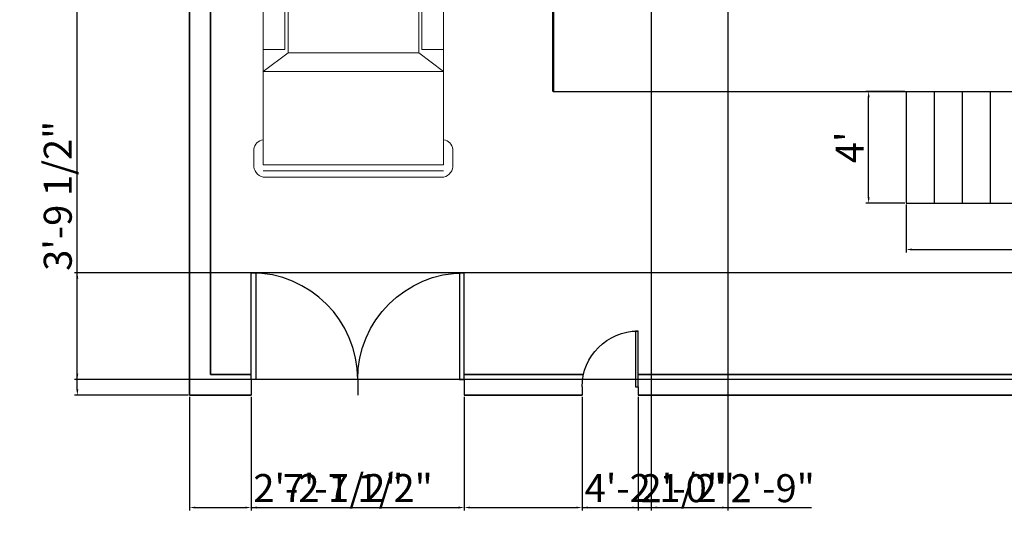
# Model space of a CAD drawing. Units: inches. Extents: x 6286 to 7213, y 5725 to 6776.
# Tile 1 of 5: x 6286 to 6709, y 5725 to 5946. Entities that reach past the tile are written whole.
import ezdxf

# ---------------------------------------------------------------- set-up
doc = ezdxf.new("R2010")
doc.units = ezdxf.units.IN
for name, color, linetype, lineweight in [('A-ANNO-DIMS', 2, 'Continuous', 18), ('A-FLOR', 7, 'Continuous', 25), ('A-FLOR-STRS', 7, 'Continuous', 25), ('A-WALL', 7, 'Continuous', 50), ('C-PKNG-VEHI', 8, 'Continuous', 13), ('C-PROP', 7, 'Continuous', 35), ('L-SITE-GATE', 3, 'Continuous', 25)]:
    doc.layers.add(name, color=color, linetype=linetype, lineweight=lineweight)
doc.styles.get("Standard").update_dxf_attribs({"font": 'arial.ttf'})
doc.dimstyles.new('ISO-25', dxfattribs={"dimtxt": 12, "dimasz": 2.5, "dimexe": 1.25, "dimexo": 0.625, "dimtad": 1, "dimdec": 1, "dimlunit": 4, "dimtxsty": 'Standard', "dimcen": 2.5, "dimadec": 0, "dimazin": 0, "dimtfac": 1, "dimtdec": 1, "dimtmove": 0, "dimatfit": 3, "dimfxl": 1, "dimarcsym": 0})

# ---------------------------------------------------------------- blocks, each defined once
blk = doc.blocks.new('*D19')
at = {"layer": 'A-ANNO-DIMS', "color": 0, "lineweight": -2, "transparency": 16777216}
for p, q in [((6665.8, 5915.26), (6649.05, 5915.26)), ((6650.3, 5869.76), (6650.3, 5912.76)), ((6665.8, 5867.26), (6649.05, 5867.26))]:
    blk.add_line(p, q, dxfattribs=at)
at = {"layer": 'A-ANNO-DIMS', "color": 0, "lineweight": 100, "transparency": 16777216}
for points in [[(6649.89, 5912.76), (6650.72, 5912.76), (6650.3, 5915.26)], [(6649.89, 5869.76), (6650.72, 5869.76), (6650.3, 5867.26)]]:
    blk.add_solid(points, dxfattribs=at)
at = {"layer": 'Defpoints', "color": 0, "lineweight": 100, "transparency": 16777216}
for p in [(6650.3, 5915.26), (6666.42, 5915.26), (6666.42, 5867.26)]:
    blk.add_point(p, dxfattribs=at)
at = {"layer": 'A-ANNO-DIMS', "color": 0, "transparency": 16777216, "insert": (6643.68, 5891.26), "char_height": 12, "attachment_point": 5, "rotation": 90}
blk.add_mtext("4'", dxfattribs=at)
blk = doc.blocks.new('*D20')
at = {"layer": 'A-ANNO-DIMS', "color": 0, "lineweight": -2, "transparency": 16777216}
for p, q in [((6666.42, 5866.64), (6666.42, 5846.12)), ((6882.42, 5866.64), (6882.42, 5846.12)), ((6668.92, 5847.37), (6879.92, 5847.37))]:
    blk.add_line(p, q, dxfattribs=at)
at = {"layer": 'A-ANNO-DIMS', "color": 0, "lineweight": 100, "transparency": 16777216}
for points in [[(6668.92, 5847.78), (6668.92, 5846.95), (6666.42, 5847.37)], [(6879.92, 5847.78), (6879.92, 5846.95), (6882.42, 5847.37)]]:
    blk.add_solid(points, dxfattribs=at)
at = {"layer": 'Defpoints', "color": 0, "lineweight": 100, "transparency": 16777216}
for p in [(6666.42, 5867.26), (6882.42, 5867.26), (6882.42, 5847.37)]:
    blk.add_point(p, dxfattribs=at)
at = {"layer": 'A-ANNO-DIMS', "color": 0, "transparency": 16777216, "insert": (6774.42, 5854.12), "char_height": 12, "attachment_point": 5}
blk.add_mtext("18'", dxfattribs=at)
blk = doc.blocks.new('*U28')
for p, q in [((5.44, 42.31), (12.12, 42.31)), ((189.69, 42.31), (183.01, 42.31)), ((0.1, -0.41), (0.1, 38.35)), ((2.77, -0.41), (2.77, 38.31)), ((5.44, -0.41), (5.44, 38.24)), ((5.45, 38.31), (16.12, 38.31)), ((16.12, 38.31), (180.34, 38.31)), ((61.52, -0.41), (61.52, 38.31)), ((61.52, 38.31), (77.54, 27.62)), ((64.19, 38.31), (76.2, 30.29)), ((76.2, 30.29), (76.2, 38.31)), ((78.87, 38.31), (78.87, 28.96)), ((106.91, 28.96), (106.91, 38.31)), ((109.58, 27.62), (109.58, 38.31)), ((112.25, 38.31), (112.25, 28.96)), ((140.29, 28.96), (140.29, 38.31)), ((141.62, 27.62), (149.64, 38.31)), ((149.64, -0.41), (149.64, 38.31)), ((189.69, 38.31), (179.01, 38.31)), ((189.69, -0.41), (189.69, 38.24)), ((192.36, -0.41), (192.36, 38.31)), ((195.03, -0.41), (195.03, 38.35)), ((77.54, 27.62), (141.62, 27.62)), ((77.54, -0.41), (77.54, 27.62)), ((78.87, 28.96), (106.91, 28.96)), ((112.25, 28.96), (140.29, 28.96)), ((141.62, -0.41), (141.62, 27.62)), ((5.44, 7.6), (61.52, 15.61)), ((0.1, -0.42), (0.1, -39.18)), ((2.77, -0.41), (2.77, -39.13)), ((5.44, -0.42), (5.44, -39.07)), ((61.52, -0.41), (61.52, -39.13)), ((77.54, -0.41), (77.54, -28.45)), ((141.62, -0.41), (141.62, -28.45)), ((149.64, -0.41), (149.64, -39.13)), ((189.69, -0.42), (189.69, -39.07)), ((192.36, -0.41), (192.36, -39.13)), ((195.03, -0.42), (195.03, -39.18)), ((5.44, -8.42), (61.52, -16.43)), ((61.52, -39.13), (77.54, -28.45)), ((77.54, -28.45), (141.62, -28.45)), ((109.58, -28.45), (109.58, -39.13)), ((141.62, -28.45), (149.64, -39.13)), ((64.19, -39.13), (76.2, -31.12)), ((76.2, -31.12), (76.2, -39.13)), ((78.87, -39.13), (78.87, -29.79)), ((78.87, -29.79), (106.91, -29.79)), ((106.91, -29.79), (106.91, -39.13)), ((112.25, -29.79), (140.29, -29.79)), ((112.25, -39.13), (112.25, -29.79)), ((140.29, -29.79), (140.29, -39.13)), ((5.45, -39.13), (16.12, -39.13)), ((16.12, -39.13), (180.34, -39.13)), ((189.69, -39.13), (179.01, -39.13)), ((5.44, -43.14), (12.12, -43.14)), ((189.69, -43.14), (183.01, -43.14))]:
    blk.add_line(p, q)
for centre, radius, start, end in [((5.06, 37.26), 5.06, 85.6455, 168.0943), ((11.45, 37.64), 4.72, 8.1301, 81.87), ((183.68, 37.64), 4.72, 98.13, 171.8699), ((190.07, 37.26), 5.06, 11.9057, 94.3545), ((5.06, -38.09), 5.06, 191.9057, 274.3545), ((11.45, -38.46), 4.72, 278.13, 351.8699), ((183.68, -38.46), 4.72, 188.1301, 261.87), ((190.07, -38.09), 5.06, 265.6455, 348.0943)]:
    blk.add_arc(centre, radius, start, end)
blk = doc.blocks.new('*U2')
for p, q in [((0, 0), (0, -6)), ((40, 0), (40, -6))]:
    blk.add_line(p, q)
blk.add_lwpolyline([(0, 0), (0, 40), (1.75, 40), (1.75, 0)], close=True)
blk.add_arc((0, 0), 40, 0, 90)
blk = doc.blocks.new('*D56')
at = {"layer": 'A-ANNO-DIMS', "color": 0, "lineweight": -2, "transparency": 16777216}
for p, q in [((6358.3, 6713.26), (6309.47, 6713.26)), ((6310.72, 5787.26), (6310.72, 6710.76)), ((6358.3, 5784.76), (6309.47, 5784.76))]:
    blk.add_line(p, q, dxfattribs=at)
at = {"layer": 'A-ANNO-DIMS', "color": 0, "lineweight": 100, "transparency": 16777216}
for points in [[(6310.31, 6710.76), (6311.14, 6710.76), (6310.72, 6713.26)], [(6310.31, 5787.26), (6311.14, 5787.26), (6310.72, 5784.76)]]:
    blk.add_solid(points, dxfattribs=at)
at = {"layer": 'Defpoints', "color": 0, "lineweight": 100, "transparency": 16777216}
for p in [(6310.72, 6713.26), (6358.92, 6713.26), (6358.92, 5784.76)]:
    blk.add_point(p, dxfattribs=at)
at = {"layer": 'A-ANNO-DIMS', "color": 0, "transparency": 16777216, "insert": (6303.89, 6249.01), "char_height": 12, "attachment_point": 5, "rotation": 90}
blk.add_mtext('77\'-4 1/2"', dxfattribs=at)
blk = doc.blocks.new('*D58')
at = {"layer": 'A-ANNO-DIMS', "color": 0, "lineweight": -2, "transparency": 16777216}
for p, q in [((6358.92, 5784.14), (6358.92, 5735.31)), ((6385.29, 5784.14), (6385.29, 5735.31)), ((6361.42, 5736.56), (6382.79, 5736.56)), ((6385.29, 5736.56), (6449.11, 5736.56))]:
    blk.add_line(p, q, dxfattribs=at)
at = {"layer": 'A-ANNO-DIMS', "color": 0, "lineweight": 100, "transparency": 16777216}
for points in [[(6361.42, 5736.98), (6361.42, 5736.15), (6358.92, 5736.56)], [(6382.79, 5736.98), (6382.79, 5736.15), (6385.29, 5736.56)]]:
    blk.add_solid(points, dxfattribs=at)
at = {"layer": 'Defpoints', "color": 0, "lineweight": 100, "transparency": 16777216}
for p in [(6358.92, 5784.76), (6385.29, 5784.76), (6385.29, 5736.56)]:
    blk.add_point(p, dxfattribs=at)
at = {"layer": 'A-ANNO-DIMS', "color": 0, "transparency": 16777216, "insert": (6418.45, 5743.39), "char_height": 12, "attachment_point": 5}
blk.add_mtext('2\'-2 1/2"', dxfattribs=at)
blk = doc.blocks.new('*D59')
at = {"layer": 'A-ANNO-DIMS', "color": 0, "lineweight": -2, "transparency": 16777216}
for p, q in [((6385.29, 5784.14), (6385.29, 5735.31)), ((6476.78, 5784.14), (6476.78, 5735.31)), ((6387.79, 5736.56), (6474.28, 5736.56))]:
    blk.add_line(p, q, dxfattribs=at)
at = {"layer": 'A-ANNO-DIMS', "color": 0, "lineweight": 100, "transparency": 16777216}
for points in [[(6387.79, 5736.98), (6387.79, 5736.15), (6385.29, 5736.56)], [(6474.28, 5736.98), (6474.28, 5736.15), (6476.78, 5736.56)]]:
    blk.add_solid(points, dxfattribs=at)
at = {"layer": 'Defpoints', "color": 0, "lineweight": 100, "transparency": 16777216}
for p in [(6385.29, 5784.76), (6476.78, 5784.76), (6476.78, 5736.56)]:
    blk.add_point(p, dxfattribs=at)
at = {"layer": 'A-ANNO-DIMS', "color": 0, "transparency": 16777216, "insert": (6431.04, 5743.39), "char_height": 12, "attachment_point": 5}
blk.add_mtext('7\'-7 1/2"', dxfattribs=at)
blk = doc.blocks.new('*D60')
at = {"layer": 'A-ANNO-DIMS', "color": 0, "lineweight": -2, "transparency": 16777216}
for p, q in [((6476.78, 5784.14), (6476.78, 5735.31)), ((6527.33, 5784.14), (6527.33, 5735.31)), ((6479.28, 5736.56), (6524.83, 5736.56)), ((6527.33, 5736.56), (6591.42, 5736.56))]:
    blk.add_line(p, q, dxfattribs=at)
at = {"layer": 'A-ANNO-DIMS', "color": 0, "lineweight": 100, "transparency": 16777216}
for points in [[(6479.28, 5736.98), (6479.28, 5736.15), (6476.78, 5736.56)], [(6524.83, 5736.98), (6524.83, 5736.15), (6527.33, 5736.56)]]:
    blk.add_solid(points, dxfattribs=at)
at = {"layer": 'Defpoints', "color": 0, "lineweight": 100, "transparency": 16777216}
for p in [(6476.78, 5784.76), (6527.33, 5784.76), (6527.33, 5736.56)]:
    blk.add_point(p, dxfattribs=at)
at = {"layer": 'A-ANNO-DIMS', "color": 0, "transparency": 16777216, "insert": (6560.63, 5743.39), "char_height": 12, "attachment_point": 5}
blk.add_mtext('4\'-2 1/2"', dxfattribs=at)
blk = doc.blocks.new('*D61')
at = {"layer": 'A-ANNO-DIMS', "color": 0, "lineweight": -2, "transparency": 16777216}
for p, q in [((6527.33, 5784.14), (6527.33, 5735.31)), ((6551.33, 5784.14), (6551.33, 5735.31)), ((6529.83, 5736.56), (6548.83, 5736.56)), ((6551.33, 5736.56), (6587.18, 5736.56))]:
    blk.add_line(p, q, dxfattribs=at)
at = {"layer": 'A-ANNO-DIMS', "color": 0, "lineweight": 100, "transparency": 16777216}
for points in [[(6529.83, 5736.98), (6529.83, 5736.15), (6527.33, 5736.56)], [(6548.83, 5736.98), (6548.83, 5736.15), (6551.33, 5736.56)]]:
    blk.add_solid(points, dxfattribs=at)
at = {"layer": 'Defpoints', "color": 0, "lineweight": 100, "transparency": 16777216}
for p in [(6527.33, 5784.76), (6551.33, 5784.76), (6551.33, 5736.56)]:
    blk.add_point(p, dxfattribs=at)
at = {"layer": 'A-ANNO-DIMS', "color": 0, "transparency": 16777216, "insert": (6570.51, 5743.32), "char_height": 12, "attachment_point": 5}
blk.add_mtext('2\'-0"', dxfattribs=at)
blk = doc.blocks.new('*D70')
at = {"layer": 'A-ANNO-DIMS', "color": 0, "lineweight": -2, "transparency": 16777216}
for p, q in [((6556.96, 6136.41), (6556.96, 5735.31)), ((6589.92, 6126.44), (6589.92, 5735.31)), ((6559.46, 5736.56), (6587.42, 5736.56)), ((6589.92, 5736.56), (6625.78, 5736.56))]:
    blk.add_line(p, q, dxfattribs=at)
at = {"layer": 'A-ANNO-DIMS', "color": 0, "lineweight": 100, "transparency": 16777216}
for points in [[(6559.46, 5736.98), (6559.46, 5736.15), (6556.96, 5736.56)], [(6587.42, 5736.98), (6587.42, 5736.15), (6589.92, 5736.56)]]:
    blk.add_solid(points, dxfattribs=at)
at = {"layer": 'Defpoints', "color": 0, "lineweight": 100, "transparency": 16777216}
for p in [(6556.96, 6137.04), (6589.92, 6127.07), (6589.92, 5736.56)]:
    blk.add_point(p, dxfattribs=at)
at = {"layer": 'A-ANNO-DIMS', "color": 0, "transparency": 16777216, "insert": (6609.1, 5743.32), "char_height": 12, "attachment_point": 5}
blk.add_mtext('2\'-9"', dxfattribs=at)
blk = doc.blocks.new('*D74')
at = {"layer": 'A-ANNO-DIMS', "color": 0, "lineweight": -2, "transparency": 16777216}
for p, q in [((6310.72, 5837.37), (6310.72, 5900.97)), ((6950.65, 5837.37), (6309.47, 5837.37)), ((6310.72, 5794.12), (6310.72, 5834.87)), ((6950.65, 5791.62), (6309.47, 5791.62))]:
    blk.add_line(p, q, dxfattribs=at)
at = {"layer": 'A-ANNO-DIMS', "color": 0, "lineweight": 100, "transparency": 16777216}
for points in [[(6310.31, 5834.87), (6311.14, 5834.87), (6310.72, 5837.37)], [(6310.31, 5794.12), (6311.14, 5794.12), (6310.72, 5791.62)]]:
    blk.add_solid(points, dxfattribs=at)
at = {"layer": 'Defpoints', "color": 0, "lineweight": 100, "transparency": 16777216}
for p in [(6310.72, 5837.37), (6951.28, 5837.37), (6951.28, 5791.62)]:
    blk.add_point(p, dxfattribs=at)
at = {"layer": 'A-ANNO-DIMS', "color": 0, "transparency": 16777216, "insert": (6303.89, 5870.42), "char_height": 12, "attachment_point": 5, "rotation": 90}
blk.add_mtext('3\'-9 1/2"', dxfattribs=at)

msp = doc.modelspace()

# ---------------------------------------------------------------- linework, layer by layer
at = {"layer": 'A-FLOR'}
msp.add_line((6514.92, 5915.26), (6738.42, 5915.26), dxfattribs=at)
at = {"layer": 'A-FLOR-STRS'}
for p, q in [((6666.42, 5915.26), (6666.42, 5867.26)), ((6678.42, 5915.26), (6678.42, 5867.26)), ((6690.42, 5915.26), (6690.42, 5867.26)), ((6702.42, 5915.26), (6702.42, 5867.26)), ((6666.42, 5867.26), (6882.42, 5867.26))]:
    msp.add_line(p, q, dxfattribs=at)
at = {"layer": 'A-WALL'}
msp.add_line((6514.92, 6194.26), (6514.92, 5915.26), dxfattribs=at)
at = {"layer": 'C-PROP'}
for p, q in [((6358.92, 6713.26), (6358.92, 5784.76)), ((6367.92, 6596.26), (6367.92, 5793.76)), ((6367.92, 5793.76), (6385.29, 5793.76)), ((6430.99, 5793.76), (6431.09, 5793.76)), ((6476.78, 5793.76), (6527.95, 5793.76)), ((6551.33, 5793.76), (6951.28, 5793.76)), ((6358.92, 5784.76), (6385.29, 5784.76)), ((6476.78, 5784.76), (6527.33, 5784.76)), ((6551.33, 5784.76), (6951.28, 5784.76))]:
    msp.add_line(p, q, dxfattribs=at)

# ---------------------------------------------------------------- block references
at = {"layer": 'C-PKNG-VEHI', "rotation": 270}
msp.add_blockref('*U28', (6429.61, 6073.49), dxfattribs=at)
at = {"layer": 'L-SITE-GATE'}
for p, xscale, yscale, zscale in [((6385.29, 5791.62), 1.143562652288551, 1.143562652288551, 1.143562652288551), ((6476.78, 5791.62), -1.143562652288551, 1.143562652288551, 1.143562652288551), ((6551.33, 5788.36), -0.5999999999999864, 0.5999999999999864, 0.5999999999999864)]:
    msp.add_blockref('*U2', p, dxfattribs=dict(at, xscale=xscale, yscale=yscale, zscale=zscale))

# ---------------------------------------------------------------- dimensions: what is measured, and where the dimension line sits
at = {"layer": 'A-ANNO-DIMS'}
for base, p1, p2, override, picture, middle in [((6310.72, 6713.26), (6358.92, 5784.76), (6358.92, 6713.26), {"dimdec": 1, "dimlfac": 1, "dimrnd": 0, "dimzin": 1, "dimdsep": 46, "dimlunit": 4, "dimfrac": 2}, '*D56', (6303.89, 6249.01)), ((6650.3, 5915.26), (6666.42, 5867.26), (6666.42, 5915.26), {"dimclrd": 0, "dimclre": 0, "dimclrt": 0}, '*D19', (6643.68, 5891.26)), ((6310.724, 5837.3674), (6951.2781, 5791.6249), (6951.2781, 5837.3674), {"dimdec": 1, "dimlfac": 1, "dimrnd": 0, "dimzin": 1, "dimdsep": 46, "dimlunit": 4, "dimfrac": 2}, '*D74', (6303.8902, 5870.4187))]:
    dim = msp.add_linear_dim(base=base, p1=p1, p2=p2, angle=90, dimstyle='ISO-25', override=override, dxfattribs=at)
    dim.commit()
    dim.dimension.update_dxf_attribs({"geometry": picture, "text_midpoint": middle})
for base, p1, p2, override, picture, middle in [((6589.92, 5736.56), (6556.96, 6137.04), (6589.92, 6127.07), {"dimdec": 1, "dimlfac": 1, "dimrnd": 0, "dimzin": 1, "dimdsep": 46, "dimlunit": 4, "dimfrac": 2}, '*D70', (6609.1, 5743.32)), ((6882.42, 5847.37), (6666.42, 5867.26), (6882.42, 5867.26), {"dimclrd": 0, "dimclre": 0, "dimclrt": 0}, '*D20', (6774.42, 5854.12)), ((6385.29, 5736.56), (6358.92, 5784.76), (6385.29, 5784.76), {"dimdec": 1, "dimlfac": 1, "dimrnd": 0, "dimzin": 1, "dimdsep": 46, "dimlunit": 4, "dimfrac": 2}, '*D58', (6418.45, 5743.39)), ((6476.78, 5736.56), (6385.29, 5784.76), (6476.78, 5784.76), {"dimdec": 1, "dimlfac": 1, "dimrnd": 0, "dimzin": 1, "dimdsep": 46, "dimlunit": 4, "dimfrac": 2}, '*D59', (6431.04, 5743.39)), ((6527.3299, 5736.5635), (6476.7784, 5784.7635), (6527.3299, 5784.7635), {"dimdec": 1, "dimlfac": 1, "dimrnd": 0, "dimzin": 1, "dimdsep": 46, "dimlunit": 4, "dimfrac": 2}, '*D60', (6560.6268, 5743.3931)), ((6551.33, 5736.56), (6527.33, 5784.76), (6551.33, 5784.76), {"dimdec": 1, "dimlfac": 1, "dimrnd": 0, "dimzin": 1, "dimdsep": 46, "dimlunit": 4, "dimfrac": 2}, '*D61', (6570.51, 5743.32))]:
    dim = msp.add_linear_dim(base=base, p1=p1, p2=p2, dimstyle='ISO-25', override=override, dxfattribs=at)
    dim.commit()
    dim.dimension.update_dxf_attribs({"geometry": picture, "text_midpoint": middle})

doc.saveas('drawing.dxf')
